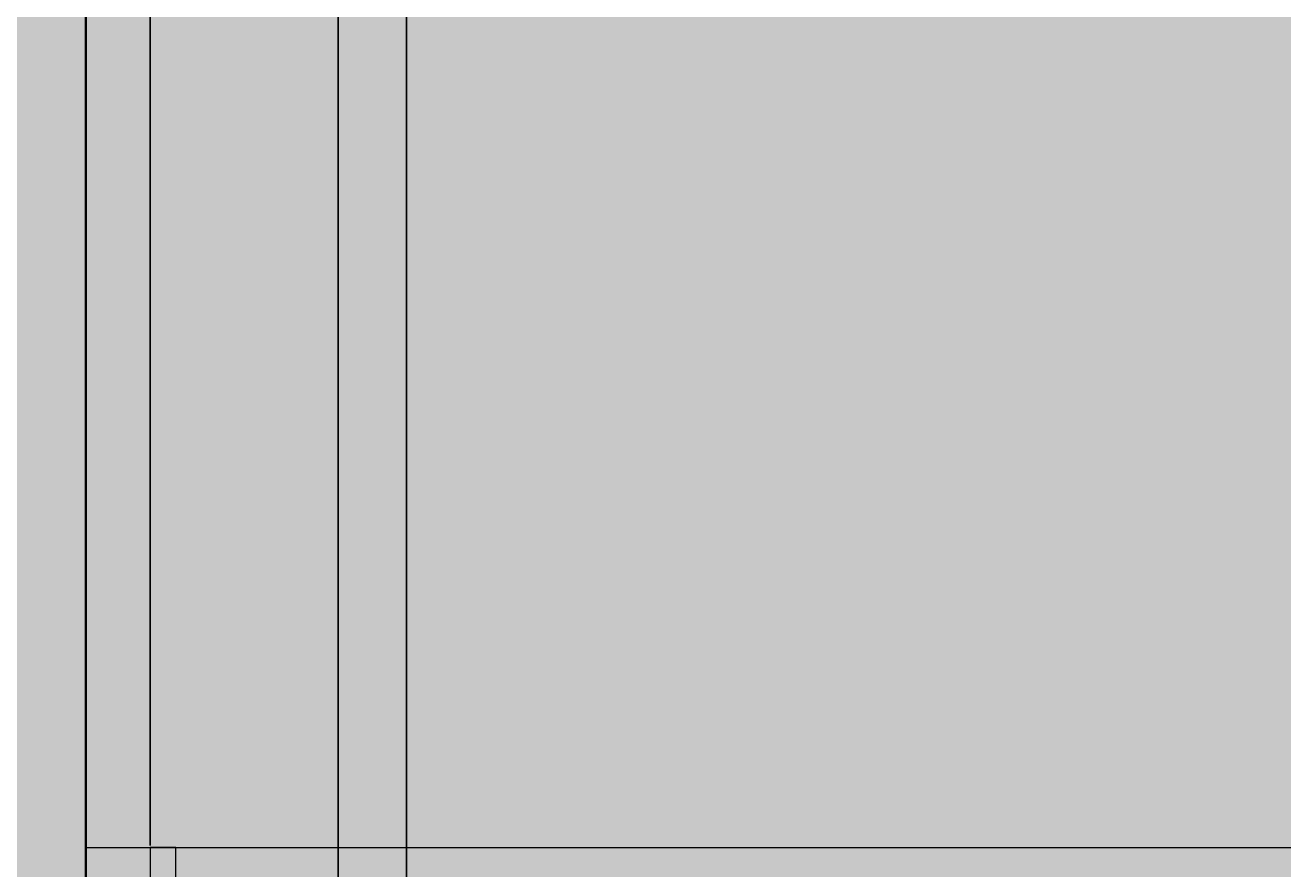
# Model space of a CAD drawing. Units: feet. Extents: x 2695 to 2912, y 795 to 1139.
# Tile 53 of 83: x 2769 to 2806, y 971 to 996. Entities that reach past the tile are written whole.
import ezdxf

# ---------------------------------------------------------------- set-up
doc = ezdxf.new("R2010")
doc.units = ezdxf.units.FT
for name, color, linetype, lineweight in [('A-ANNO-DIMS', 2, 'Continuous', 18), ('A-ELEV', 7, 'Continuous', 35), ('A-ELEV-PATT', 252, 'Continuous', 13), ('A-ELEV-RAIL', 8, 'Continuous', 18), ('A-GLAZ', 4, 'Continuous', 25), ('A-GLAZ-PATT', 254, 'Continuous', 13)]:
    doc.layers.add(name, color=color, linetype=linetype, lineweight=lineweight)
doc.styles.get("Standard").update_dxf_attribs({"font": 'arial.ttf'})
doc.dimstyles.get("Standard").update_dxf_attribs({"dimtxt": 0.18, "dimasz": 0.18, "dimexe": 0.18, "dimexo": 0.0625, "dimgap": 0.09, "dimtad": 0, "dimtih": 1, "dimtoh": 1, "dimdec": 1, "dimzin": 0, "dimdsep": 46, "dimlunit": 3, "dimtxsty": 'Standard', "dimcen": 0.09, "dimadec": 0, "dimazin": 0, "dimtfac": 1, "dimtdec": 1, "dimtofl": 0, "dimtmove": 0, "dimatfit": 3, "dimfxl": 1, "dimtolj": 1, "dimtzin": 0, "dimarcsym": 0})

# ---------------------------------------------------------------- blocks, each defined once
blk = doc.blocks.new('*D48')
at = {"layer": 'A-ANNO-DIMS', "color": 0, "lineweight": -2, "transparency": 16777216}
for p, q in [((2770.636, 972.03), (2770.636, 1138.886)), ((2770.816, 1138.706), (2771.263, 1138.706)), ((2772.342, 1138.706), (2771.894, 1138.706)), ((2772.522, 972.03), (2772.522, 1138.886))]:
    blk.add_line(p, q, dxfattribs=at)
at = {"layer": 'A-ANNO-DIMS', "color": 0, "transparency": 16777216}
for points in [[(2770.816, 1138.736), (2770.816, 1138.676), (2770.636, 1138.706)], [(2772.342, 1138.736), (2772.342, 1138.676), (2772.522, 1138.706)]]:
    blk.add_solid(points, dxfattribs=at)
at = {"layer": 'Defpoints', "color": 0, "transparency": 16777216}
for p in [(2772.522, 1138.706), (2770.636, 971.967), (2772.522, 971.967)]:
    blk.add_point(p, dxfattribs=at)
at = {"layer": 'A-ANNO-DIMS', "color": 0, "transparency": 16777216, "insert": (2771.579, 1138.706), "char_height": 0.18, "attachment_point": 5}
blk.add_mtext('\\A1;1.89', dxfattribs=at)
blk = doc.blocks.new('*D49')
at = {"layer": 'A-ANNO-DIMS', "color": 0, "lineweight": -2, "transparency": 16777216}
for p, q in [((2772.522, 972.03), (2772.522, 1138.886)), ((2772.702, 1138.706), (2790.888, 1138.706)), ((2809.861, 1138.706), (2791.674, 1138.706)), ((2810.041, 972.03), (2810.041, 1138.886))]:
    blk.add_line(p, q, dxfattribs=at)
at = {"layer": 'A-ANNO-DIMS', "color": 0, "transparency": 16777216}
for points in [[(2772.702, 1138.736), (2772.702, 1138.676), (2772.522, 1138.706)], [(2809.861, 1138.736), (2809.861, 1138.676), (2810.041, 1138.706)]]:
    blk.add_solid(points, dxfattribs=at)
at = {"layer": 'Defpoints', "color": 0, "transparency": 16777216}
for p in [(2810.041, 1138.706), (2772.522, 971.967), (2810.041, 971.967)]:
    blk.add_point(p, dxfattribs=at)
at = {"layer": 'A-ANNO-DIMS', "color": 0, "transparency": 16777216, "insert": (2791.281, 1138.706), "char_height": 0.18, "attachment_point": 5}
blk.add_mtext('\\A1;37.52', dxfattribs=at)

msp = doc.modelspace()

# ---------------------------------------------------------------- hatches: boundary and pattern name
at = {"layer": 'A-ELEV-PATT'}
h = msp.add_hatch(color=256, dxfattribs=at)
h.set_gradient(color1=(147, 149, 152), color2=(147, 149, 152), tint=1)
h.paths.add_polyline_path([(2770.6361, 1118.4096), (2710.6361, 1118.4096), (2710.6361, 1062.9306), (2770.6361, 1062.9306)])
h.paths.add_polyline_path([(2890.6361, 1103.3378), (2770.6361, 1103.3378), (2770.6361, 1062.9306), (2890.6361, 1062.9306)])
h.paths.add_polyline_path([(2730.7081, 1048.1052), (2755.1125, 1048.1052), (2755.1125, 936.9306), (2770.6361, 936.9306), (2770.6361, 1050.3105), (2715.8852, 1050.3105), (2715.8852, 936.9306), (2730.7081, 936.9306)])
h.paths.add_polyline_path([(2890.6361, 1050.3105), (2770.6361, 1050.3105), (2770.6361, 971.9673), (2778.0341, 971.9673), (2778.0341, 1020.8235), (2843.575, 1020.8235), (2843.575, 971.9673), (2890.6361, 971.9673)])
h.paths.add_polyline_path([(2888.1882, 970.7156), (2843.575, 970.7156), (2843.575, 964.8267), (2888.1882, 964.8267)])
h.paths.add_polyline_path([(2888.1882, 964.1328), (2843.575, 964.1328), (2843.575, 956.614), (2888.1882, 956.614)])
h.paths.add_polyline_path([(2888.1882, 955.9202), (2843.575, 955.9202), (2843.575, 949.2892), (2888.1882, 949.2892)])
h.paths.add_polyline_path([(2888.1882, 948.5954), (2843.575, 948.5954), (2843.575, 941.3507), (2888.1882, 941.3507)])
h.paths.add_polyline_path([(2888.1882, 940.6569), (2843.575, 940.6569), (2843.575, 936.9306), (2888.1882, 936.9306)])
h.paths.add_polyline_path([(2890.6361, 970.7156), (2888.9368, 970.7156), (2888.9368, 964.8267), (2890.6361, 964.8267)])
h.paths.add_polyline_path([(2890.6361, 964.1328), (2888.9368, 964.1328), (2888.9368, 956.614), (2890.6361, 956.614)])
h.paths.add_polyline_path([(2890.6361, 955.9202), (2888.9368, 955.9202), (2888.9368, 949.2892), (2890.6361, 949.2892)])
h.paths.add_polyline_path([(2890.6361, 940.6569), (2888.9368, 940.6569), (2888.9368, 936.9306), (2890.6361, 936.9306)])
h.paths.add_polyline_path([(2890.6361, 948.5954), (2888.9368, 948.5954), (2888.9368, 941.3507), (2890.6361, 941.3507)])
h.paths.add_polyline_path([(2772.5216, 970.7156), (2770.6361, 970.7156), (2770.6361, 964.8267), (2772.5216, 964.8267)])
h.paths.add_polyline_path([(2772.5216, 964.1328), (2770.6361, 964.1328), (2770.6361, 956.614), (2772.5216, 956.614)])
h.paths.add_polyline_path([(2772.5216, 955.9202), (2770.6361, 955.9202), (2770.6361, 949.2892), (2772.5216, 949.2892)])
h.paths.add_polyline_path([(2772.5216, 948.5954), (2770.6361, 948.5954), (2770.6361, 941.3507), (2772.5216, 941.3507)])
h.paths.add_polyline_path([(2772.5216, 940.6569), (2770.6361, 940.6569), (2770.6361, 936.9306), (2772.5216, 936.9306)])
h.paths.add_polyline_path([(2778.0341, 940.6569), (2773.2702, 940.6569), (2773.2702, 936.9306), (2778.0341, 936.9306)])
h.paths.add_polyline_path([(2778.0341, 970.7156), (2773.2702, 970.7156), (2773.2702, 964.8267), (2778.0341, 964.8267)])
h.paths.add_polyline_path([(2778.0341, 964.1328), (2773.2702, 964.1328), (2773.2702, 956.614), (2778.0341, 956.614)])
h.paths.add_polyline_path([(2778.0341, 955.9202), (2773.2702, 955.9202), (2773.2702, 949.2892), (2778.0341, 949.2892)])
h.paths.add_polyline_path([(2778.0341, 948.5954), (2773.2702, 948.5954), (2773.2702, 941.3507), (2778.0341, 941.3507)])
h.paths.add_polyline_path([(2810.0407, 940.6569), (2780.0341, 940.6569), (2780.0341, 936.9306), (2810.0407, 936.9306)])
h.paths.add_polyline_path([(2890.6361, 924.3105), (2770.6361, 924.3105), (2770.6361, 810.9306), (2773.5029, 810.9306), (2773.5029, 905.5143), (2805.9398, 905.5143), (2838.3767, 905.5143), (2838.3767, 810.9306), (2890.6361, 810.9306)])
h = msp.add_hatch(color=256, dxfattribs=at)
h.set_gradient(color2=(0, 0, 0), tint=1)
h.paths.add_polyline_path([(2772.5216, 971.9673), (2770.6361, 971.9673), (2770.6361, 970.7156), (2772.5216, 970.7156)])
h.paths.add_polyline_path([(2773.2702, 971.9673), (2772.5216, 971.9673), (2772.5216, 970.7156), (2773.2702, 970.7156)])
h.paths.add_polyline_path([(2778.0341, 971.9673), (2773.2702, 971.9673), (2773.2702, 970.7156), (2778.0341, 970.7156)])
h.paths.add_polyline_path([(2780.0341, 971.9673), (2778.0341, 971.9673), (2778.0341, 970.7156), (2780.0341, 970.7156)])
h.paths.add_polyline_path([(2841.575, 971.9673), (2780.0341, 971.9673), (2780.0341, 970.7156), (2841.575, 970.7156)])
h.paths.add_polyline_path([(2843.575, 971.9673), (2841.575, 971.9673), (2841.575, 970.7156), (2843.575, 970.7156)])
h.paths.add_polyline_path([(2888.1882, 971.9673), (2843.575, 971.9673), (2843.575, 970.7156), (2888.1882, 970.7156)])
h.paths.add_polyline_path([(2888.9368, 971.9673), (2888.1882, 971.9673), (2888.1882, 970.7156), (2888.9368, 970.7156)], flags=17)
h.paths.add_polyline_path([(2890.6361, 971.9673), (2888.9368, 971.9673), (2888.9368, 970.7156), (2890.6361, 970.7156)])
h.paths.add_polyline_path([(2888.9368, 971.9673), (2888.1882, 971.9673), (2888.1882, 964.8267), (2888.9368, 964.8267)])
h.paths.add_polyline_path([(2888.9368, 964.8267), (2888.1882, 964.8267), (2888.1882, 964.1328), (2888.9368, 964.1328)])
h.paths.add_polyline_path([(2890.6361, 964.8267), (2888.9368, 964.8267), (2888.9368, 964.1328), (2890.6361, 964.1328)])
h.paths.add_polyline_path([(2888.1882, 964.8267), (2770.6361, 964.8267), (2770.6361, 964.1328), (2888.1882, 964.1328)])
h.paths.add_polyline_path([(2888.9368, 964.1328), (2888.1882, 964.1328), (2888.1882, 936.9306), (2888.9368, 936.9306)])
h.paths.add_polyline_path([(2890.6361, 956.614), (2888.9368, 956.614), (2888.9368, 955.9202), (2890.6361, 955.9202)])
h.paths.add_polyline_path([(2888.1882, 956.614), (2770.6361, 956.614), (2770.6361, 955.9202), (2888.1882, 955.9202)])
h.paths.add_polyline_path([(2890.6361, 949.2892), (2888.9368, 949.2892), (2888.9368, 948.5954), (2890.6361, 948.5954)])
h.paths.add_polyline_path([(2888.1882, 949.2892), (2770.6361, 949.2892), (2770.6361, 948.5954), (2888.1882, 948.5954)])
h.paths.add_polyline_path([(2890.6361, 941.3507), (2888.9368, 941.3507), (2888.9368, 940.6569), (2890.6361, 940.6569)])
h.paths.add_polyline_path([(2888.1882, 941.3507), (2770.6361, 941.3507), (2770.6361, 940.6569), (2888.1882, 940.6569)])
h.paths.add_polyline_path([(2773.2702, 970.7156), (2772.5216, 970.7156), (2772.5216, 964.8267), (2773.2702, 964.8267)])
h.paths.add_polyline_path([(2773.2702, 964.1328), (2772.5216, 964.1328), (2772.5216, 956.614), (2773.2702, 956.614)])
h.paths.add_polyline_path([(2773.2702, 955.9202), (2772.5216, 955.9202), (2772.5216, 936.9306), (2773.2702, 936.9306)])
h.paths.add_polyline_path([(2810.7893, 970.7156), (2810.0407, 970.7156), (2810.0407, 964.8267), (2810.7893, 964.8267)], flags=17)
h.paths.add_polyline_path([(2810.7893, 964.1328), (2810.0407, 964.1328), (2810.0407, 956.614), (2810.7893, 956.614)], flags=17)
h.paths.add_polyline_path([(2810.7893, 955.9202), (2810.0407, 955.9202), (2810.0407, 949.2892), (2810.7893, 949.2892)], flags=17)
h.paths.add_polyline_path([(2810.7893, 971.9673), (2810.0407, 971.9673), (2810.0407, 941.3507), (2810.7893, 941.3507)])
h.paths.add_polyline_path([(2810.7893, 940.6569), (2810.0407, 940.6569), (2810.0407, 936.9306), (2810.7893, 936.9306)])
h.paths.add_polyline_path([(2780.0341, 1018.8235), (2841.575, 1018.8235), (2841.575, 971.9673), (2843.575, 971.9673), (2843.575, 1020.8235), (2778.0341, 1020.8235), (2778.0341, 971.9673), (2780.0341, 971.9673)])
h.paths.add_polyline_path([(2780.0341, 970.7156), (2778.0341, 970.7156), (2778.0341, 964.8267), (2780.0341, 964.8267)])
h.paths.add_polyline_path([(2780.0341, 964.1328), (2778.0341, 964.1328), (2778.0341, 956.614), (2780.0341, 956.614)])
h.paths.add_polyline_path([(2780.0341, 955.9202), (2778.0341, 955.9202), (2778.0341, 949.2892), (2780.0341, 949.2892)])
h.paths.add_polyline_path([(2780.0341, 948.5954), (2778.0341, 948.5954), (2778.0341, 941.3507), (2780.0341, 941.3507)])
h.paths.add_polyline_path([(2780.0341, 940.6569), (2778.0341, 940.6569), (2778.0341, 936.9306), (2780.0341, 936.9306)])
h.paths.add_polyline_path([(2843.575, 940.6569), (2841.575, 940.6569), (2841.575, 936.9306), (2843.575, 936.9306)])
h.paths.add_polyline_path([(2843.575, 948.5954), (2841.575, 948.5954), (2841.575, 941.3507), (2843.575, 941.3507)])
h.paths.add_polyline_path([(2843.575, 970.7156), (2841.575, 970.7156), (2841.575, 964.8267), (2843.575, 964.8267)])
h.paths.add_polyline_path([(2843.575, 964.1328), (2841.575, 964.1328), (2841.575, 956.614), (2843.575, 956.614)])
h.paths.add_polyline_path([(2843.575, 955.9202), (2841.575, 955.9202), (2841.575, 949.2892), (2843.575, 949.2892)])
h.paths.add_polyline_path([(2805.0538, 874.1057), (2803.9681, 874.1057), (2803.9681, 846.2857), (2805.0538, 846.2857)])
h.paths.add_polyline_path([(2758.1515, 902.577), (2724.1893, 902.577), (2724.1893, 874.8571), (2758.1515, 874.8571)])
h.paths.add_polyline_path([(2726.1893, 900.577), (2756.1515, 900.577), (2756.1515, 876.8571), (2726.1893, 876.8571)], flags=16)
h.paths.add_polyline_path([(2740.7302, 900.577), (2741.6105, 900.577), (2741.6105, 876.8571), (2740.7302, 876.8571)], flags=0)
at = {"layer": 'A-GLAZ-PATT'}
h = msp.add_hatch(color=256, dxfattribs=at)
h.set_gradient(color1=(213, 227, 240), color2=(213, 227, 240))
h.paths.add_polyline_path([(2810.8045, 1018.8235), (2780.0341, 1018.8235), (2780.0341, 971.9673), (2810.8045, 971.9673)])
h.paths.add_polyline_path([(2841.575, 1018.8235), (2810.8045, 1018.8235), (2810.8045, 971.9673), (2841.575, 971.9673)])
h.paths.add_polyline_path([(2810.0407, 970.7156), (2780.0341, 970.7156), (2780.0341, 964.8267), (2810.0407, 964.8267)])
h.paths.add_polyline_path([(2841.575, 970.7156), (2810.8045, 970.7156), (2810.8045, 964.8267), (2841.575, 964.8267)])
h.paths.add_polyline_path([(2841.575, 964.1328), (2810.8045, 964.1328), (2810.8045, 956.614), (2841.575, 956.614)])
h.paths.add_polyline_path([(2810.0407, 964.1328), (2780.0341, 964.1328), (2780.0341, 956.614), (2810.0407, 956.614)])
h.paths.add_polyline_path([(2810.0407, 955.9202), (2780.0341, 955.9202), (2780.0341, 949.2892), (2810.0407, 949.2892)])
h.paths.add_polyline_path([(2841.575, 955.9202), (2810.8045, 955.9202), (2810.8045, 949.2892), (2841.575, 949.2892)])
h.paths.add_polyline_path([(2841.575, 948.5954), (2810.8045, 948.5954), (2810.8045, 941.3507), (2841.575, 941.3507)])
h.paths.add_polyline_path([(2810.0407, 948.5954), (2780.0341, 948.5954), (2780.0341, 941.3507), (2810.0407, 941.3507)])
h.paths.add_polyline_path([(2810.0407, 940.6569), (2780.0341, 940.6569), (2780.0341, 936.9306), (2810.0407, 936.9306)])
h.paths.add_polyline_path([(2841.575, 940.6569), (2810.8045, 940.6569), (2810.8045, 936.9306), (2841.575, 936.9306)])

# ---------------------------------------------------------------- linework, layer by layer
at = {"layer": 'A-ELEV'}
msp.add_line((2770.6361, 1050.3105), (2770.6361, 936.9306), dxfattribs=at)
at = {"layer": 'A-ELEV-RAIL'}
msp.add_line((2770.6361, 971.9673), (2890.6361, 971.9673), dxfattribs=at)
msp.add_lwpolyline([(2773.2702, 971.9673), (2772.5216, 971.9673), (2772.5216, 936.9306), (2773.2702, 936.9306)], close=True, dxfattribs=at)
at = {"layer": 'A-GLAZ'}
for points in [[(2778.0341, 936.9306), (2778.0341, 1020.8235), (2843.575, 1020.8235), (2843.575, 936.9306)], [(2780.0341, 936.9306), (2780.0341, 1018.8235), (2841.575, 1018.8235), (2841.575, 936.9306)]]:
    msp.add_lwpolyline(points, dxfattribs=at)

# ---------------------------------------------------------------- dimensions: what is measured, and where the dimension line sits
at = {"layer": 'A-ANNO-DIMS'}
for base, p1, p2, picture, middle in [((2772.5216, 1138.7056), (2770.6361, 971.9673), (2772.5216, 971.9673), '*D48', (2771.5788, 1138.7056)), ((2810.0407, 1138.7056), (2772.5216, 971.9673), (2810.0407, 971.9673), '*D49', (2791.2811, 1138.7056))]:
    dim = msp.add_linear_dim(base=base, p1=p1, p2=p2, dimstyle='Standard', override={"dimdec": 2, "dimlfac": 1, "dimrnd": 0, "dimzin": 0, "dimdsep": 46, "dimlunit": 2}, dxfattribs=at)
    dim.commit()
    dim.dimension.update_dxf_attribs({"geometry": picture, "text_midpoint": middle})

doc.saveas('drawing.dxf')
